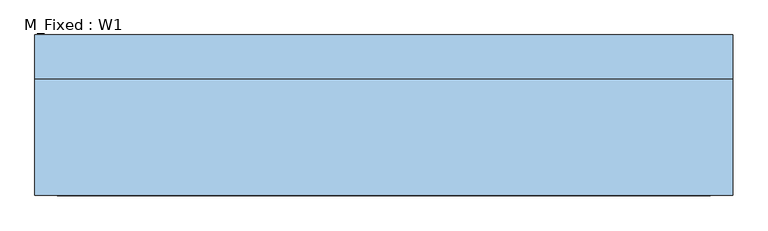
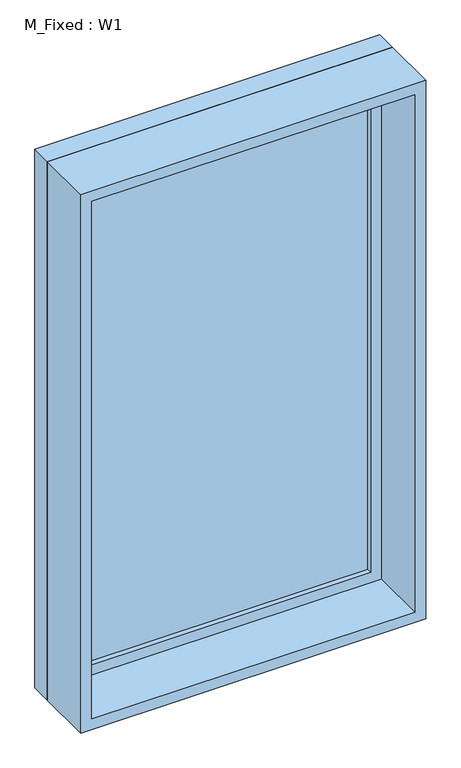
"""IFC4 building model written with IfcOpenShell, lengths in millimetres: window geometry, M_Fixed : W1."""

from ifc_helpers import new_model, si_unit, frame, origin, place, context, project, spatial, polyline, outline, extrude, source, transform, mapped, element, save


def m_fixed_w1_4c5c34d1(model_context):
    return source(origin(), model_context, "Body", "SweptSolid", [
        extrude(outline(polyline([(-437.0, 93.0), (437.0, 93.0), (437.0, 81.0), (-437.0, 81.0), (-437.0, 93.0)])), frame((0.0, 0.0, 513.0), z_axis=(0.0, 0.0, 1.0), x_axis=(1.0, 0.0, 0.0)), (0.0, 0.0, 1.0), 1524.0),
        extrude(outline(polyline([(2081.0, -481.0), (469.0, -481.0), (469.0, 481.0), (2081.0, 481.0), (2081.0, -481.0)]), holes=[polyline([(2037.0, -437.0), (2037.0, 437.0), (513.0, 437.0), (513.0, -437.0), (2037.0, -437.0)])]), frame((0.0, 65.0, 0.0), z_axis=(0.0, 1.0, 0.0), x_axis=(0.0, 0.0, 1.0)), (0.0, 0.0, 1.0), 44.0),
        extrude(outline(polyline([(2100.0, -500.0), (450.0, -500.0), (450.0, 500.0), (2100.0, 500.0), (2100.0, -500.0)]), holes=[polyline([(2081.0, -481.0), (2081.0, 481.0), (469.0, 481.0), (469.0, -481.0), (2081.0, -481.0)])]), frame((0.0, 65.0, 0.0), z_axis=(0.0, 1.0, 0.0), x_axis=(0.0, 0.0, 1.0)), (0.0, 0.0, 1.0), 63.0),
        extrude(outline(polyline([(2100.0, -500.0), (450.0, -500.0), (450.0, 500.0), (2100.0, 500.0), (2100.0, -500.0)]), holes=[polyline([(2068.0, -468.0), (2068.0, 468.0), (482.0, 468.0), (482.0, -468.0), (2068.0, -468.0)])]), frame((0.0, -102.0, 0.0), z_axis=(0.0, 1.0, 0.0), x_axis=(0.0, 0.0, 1.0)), (0.0, 0.0, 1.0), 167.0),
    ])


if __name__ == "__main__":
    model = new_model("IFC4")
    model_context = context("Model", 3, world=origin())
    ifc_project = project(units=[si_unit("LENGTHUNIT", "METRE", prefix="MILLI")], contexts=[model_context])
    site = spatial("IfcSite", under=ifc_project)
    building = spatial("IfcBuilding", under=site)
    placement = place(None, origin())
    m_fixed_w1_shape = m_fixed_w1_4c5c34d1(model_context)
    element("IfcWindow", 1, ObjectType="M_Fixed : W1", at=placement, inside=building, context=model_context, shape_type="MappedRepresentation", body=[
        mapped(m_fixed_w1_shape, transform((0.0, 0.0, 0.0), x_axis=(1.0, 0.0, 0.0), y_axis=(0.0, 1.0, 0.0), z_axis=(0.0, 0.0, 1.0))),
    ])
    save(model, "model.ifc")

# Revit data of these elements
# Type "M_Fixed : W1"
#   Type Mark = "19"
#   Height = 1650 mm
#   Default Sill Height = 450 mm
#   Width = 1000 mm
#   Window Inset = 19 mm
#   Frame Exterior Material = Iron, Ductile
#   Frame Interior Material = Iron, Ductile
#   Glass Pane Material = Glass
#   Sash = Iron, Ductile
#   Wall Closure = (empty or 0)
# Element 1 (IfcWindow, "M_Fixed : W1")
#   Materials on its faces: "Iron, Ductile", "Glass"
# Materials
#   "Iron, Ductile": class "Metal", colour RGB 90 97 102, transparency 0, Description = "Ductile cast iron", Cost = 0
#   "Glass": class "Glass", colour RGB 218 227 224, transparency 0.85, Description = "Soda Lime Glass", Cost = 0
